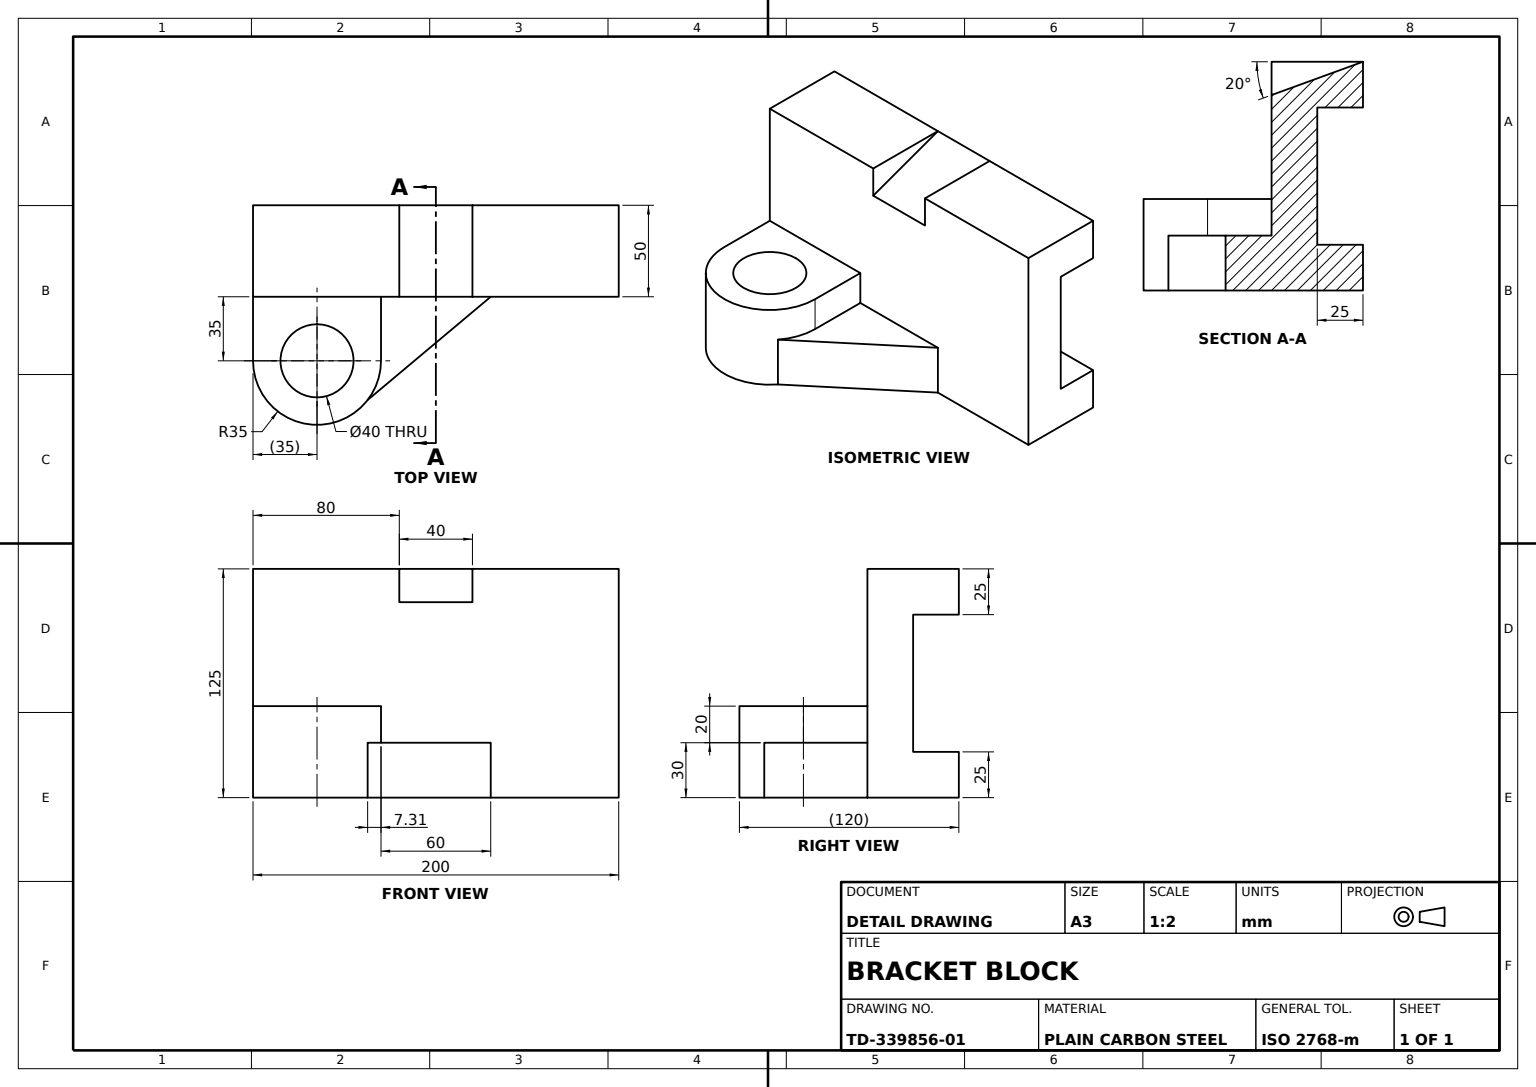
from build123d import *

# Parameters (mm, degrees)
BASE_BLOCK_SKETCH_W   = 200
BASE_BLOCK_SKETCH_H   = 125
BASE_BLOCK_DEPTH      = 50
UPPER_BLOCK_DEPTH     = 50
LUG_BOSS_DEPTH        = 30
LUG_BORE_SKETCH_R     = 20
LUG_BORE_DEPTH        = 50
CHANNEL_CUT_DEPTH     = 200
CORNER_TRIM_CUT_DEPTH = 200
TAPER_FILL_1_DEPTH    = 80
TAPER_FILL_2_DEPTH    = 80


with BuildPart() as part:
    # Base Block Sketch → Base Block (new body)
    with BuildSketch(Plane.XY):
        with Locations((100, -62.5)):
            Rectangle(BASE_BLOCK_SKETCH_W, BASE_BLOCK_SKETCH_H)
    extrude(amount=BASE_BLOCK_DEPTH)

    # Upper Block Sketch → Upper Block (add)
    with BuildSketch(Plane(origin=(0, 0, 0), x_dir=(1, 0, 0), z_dir=(0, 1, 0))):
        with BuildLine():
            Line((0, 0), (70, 0))
            Line((70, 0), (70, 35))
            ThreePointArc((70, 35), (35, 70), (0, 35))
            Line((0, 35), (0, 0))
        make_face()
    extrude(amount=-UPPER_BLOCK_DEPTH)

    # Lug Sketch → Lug Boss (add)
    with BuildSketch(Plane(origin=(0, 0, 0), x_dir=(1, 0, 0), z_dir=(0, 1, 0))):
        with BuildLine():
            Line((70, 0), (130, 0))
            Line((130, 0), (62.686080753, 56.412167861))
            ThreePointArc((62.686080753, 56.412167861), (68.121087138, 46.31342507), (70, 35))
            Line((70, 35), (70, 0))
        make_face()
    extrude(amount=-LUG_BOSS_DEPTH)

    # Lug Bore Sketch → Lug Bore (cut)
    with BuildSketch(Plane.XZ.offset(50)):
        with Locations(Location((35, -35, 0), (0, 0, 270))):
            Circle(LUG_BORE_SKETCH_R)
    extrude(amount=-LUG_BORE_DEPTH, mode=Mode.SUBTRACT)

    # Channel Sketch → Channel Cut (cut)
    with BuildSketch(Plane(origin=(200, 0, 0), x_dir=(0, 0, -1), z_dir=(1, 0, 0))):
        Polygon((-50, -62.5), (-50, -25), (-25, -25), (-25, -100), (-50, -100), align=None)
    extrude(amount=-CHANNEL_CUT_DEPTH, mode=Mode.SUBTRACT)

    # Corner Trim Sketch → Corner Trim Cut (cut)
    with BuildSketch(Plane(origin=(200, 0, 0), x_dir=(0, 0, -1), z_dir=(1, 0, 0))):
        Polygon((-50, -125), (0.050929029, -106.782951636), (0, -125), align=None)
    extrude(amount=-CORNER_TRIM_CUT_DEPTH, mode=Mode.SUBTRACT)

    # Taper Fill 1 Sketch → Taper Fill 1 (add)
    with BuildSketch(Plane(origin=(200, 0, 0), x_dir=(0, 0, -1), z_dir=(1, 0, 0))):
        Polygon((-50, -125), (0, -106.801488287), (0, -125), align=None)
    extrude(amount=-TAPER_FILL_1_DEPTH)

    # Taper Fill 2 Sketch → Taper Fill 2 (add)
    with BuildSketch(Plane.ZY):
        Polygon((0, -106.801488287), (50, -125), (0, -125), align=None)
    extrude(amount=-TAPER_FILL_2_DEPTH)


solid = part.part
